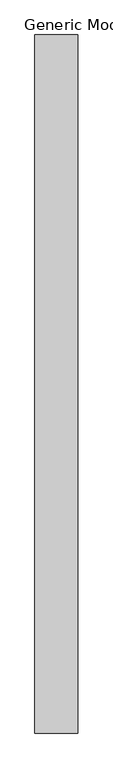
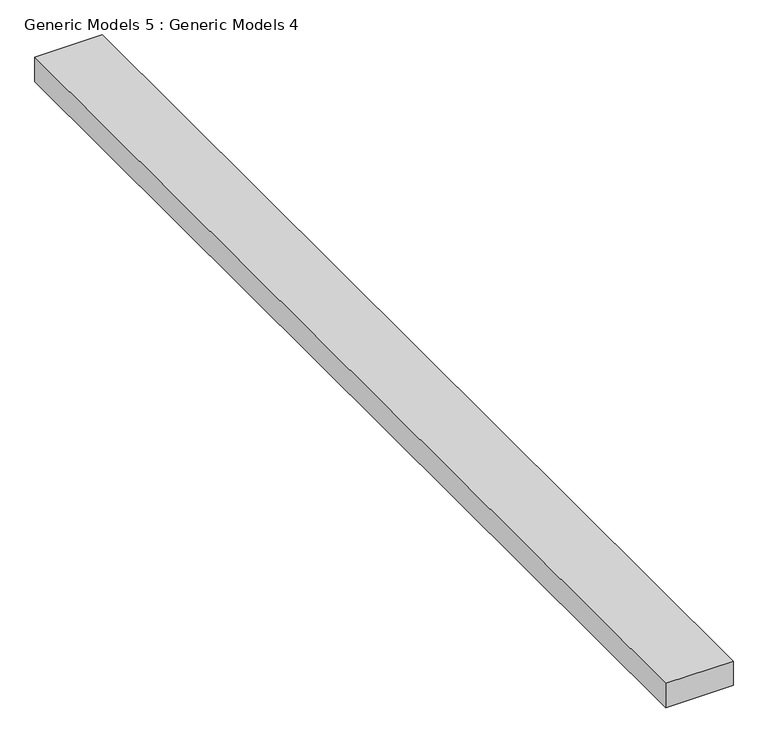
"""IFC4 building model written with IfcOpenShell, lengths in millimetres: proxy geometry, Generic Models 5 : Generic Models 4."""

from ifc_helpers import new_model, si_unit, frame, origin, place, context, project, spatial, polyline, outline, extrude, source, transform, mapped, element, save


def generic_models_5_generic_models_4_07a2a312(model_context):
    return source(origin(), model_context, "Body", "SweptSolid", [
        extrude(outline(polyline([(14902.7853663, 13.6653678), (14902.7853663, -12899.9178695), (14106.5361222, -12899.9178695), (14106.5361222, 13.6653678), (14902.7853663, 13.6653678)])), frame((0.0, 0.0, 6096.0), z_axis=(0.0, 0.0, 1.0), x_axis=(1.0, 0.0, 0.0)), (0.0, 0.0, 1.0), 304.8),
    ])


if __name__ == "__main__":
    model = new_model("IFC4")
    model_context = context("Model", 3, world=origin())
    ifc_project = project(units=[si_unit("LENGTHUNIT", "METRE", prefix="MILLI")], contexts=[model_context])
    site = spatial("IfcSite", under=ifc_project)
    building = spatial("IfcBuilding", under=site)
    placement = place(None, origin())
    generic_models_5_generic_models_4_shape = generic_models_5_generic_models_4_07a2a312(model_context)
    element("IfcBuildingElementProxy", 1, Name="Generic Models 5 : Generic Models 4", ObjectType="Generic Models 5 : Generic Models 4", at=placement, inside=building, context=model_context, shape_type="MappedRepresentation", body=[
        mapped(generic_models_5_generic_models_4_shape, transform((0.0, 0.0, 0.0), x_axis=(1.0, 0.0, 0.0), y_axis=(0.0, 1.0, 0.0), z_axis=(0.0, 0.0, 1.0))),
    ])
    save(model, "model.ifc")
